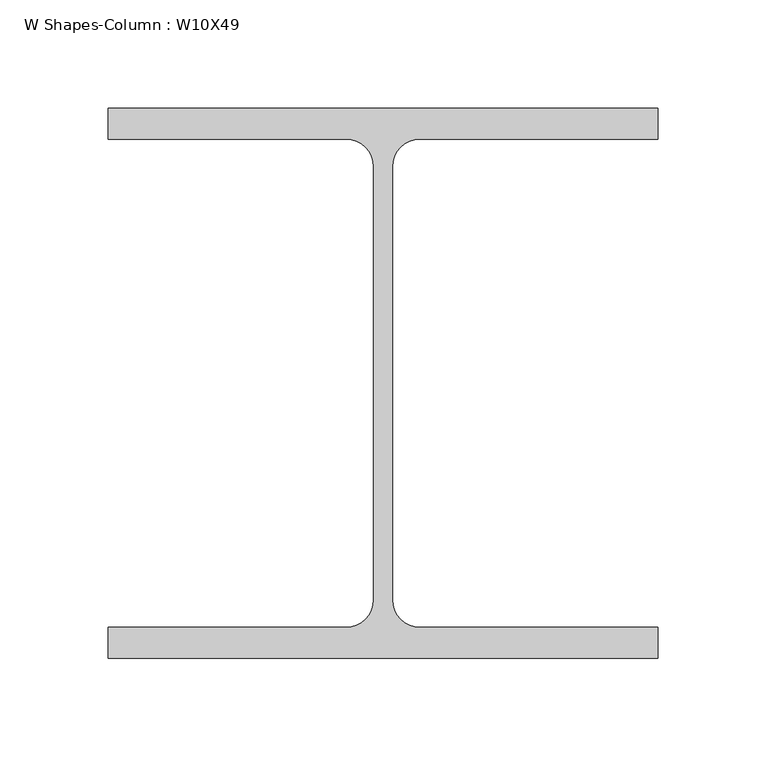
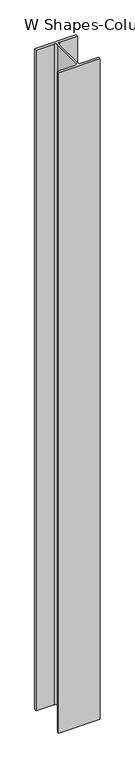
"""IFC4 building model written with IfcOpenShell, lengths in millimetres: column geometry, W Shapes-Column : W10X49."""

from ifc_helpers import new_model, si_unit, point, frame, frame_2d, origin, place, context, project, spatial, polyline, circle_curve, trimmed, segment, composite_curve, outline, extrude, source, transform, mapped, element, save


def w_shapes_column_w10x49_6b2d3d6a(model_context):
    return source(origin(), model_context, "Body", "SweptSolid", [
        extrude(outline(composite_curve([segment(polyline([(127.0, 127.0), (127.0, 112.776), (17.018, 112.776)]), True, "CONTINUOUS"), segment(trimmed(circle_curve(frame_2d((17.018, 100.076)), 12.7), [point((17.018, 112.776))], [point((4.318, 100.076))], True, "CARTESIAN"), True, "CONTINUOUS"), segment(polyline([(4.318, 100.076), (4.318, -100.076)]), True, "CONTINUOUS"), segment(trimmed(circle_curve(frame_2d((17.018, -100.076)), 12.7), [point((4.318, -100.076))], [point((17.018, -112.776))], True, "CARTESIAN"), True, "CONTINUOUS"), segment(polyline([(17.018, -112.776), (127.0, -112.776), (127.0, -127.0), (-127.0, -127.0), (-127.0, -112.776), (-17.018, -112.776)]), True, "CONTINUOUS"), segment(trimmed(circle_curve(frame_2d((-17.018, -100.076)), 12.7), [point((-17.018, -112.776))], [point((-4.318, -100.076))], True, "CARTESIAN"), True, "CONTINUOUS"), segment(polyline([(-4.318, -100.076), (-4.318, 100.076)]), True, "CONTINUOUS"), segment(trimmed(circle_curve(frame_2d((-17.018, 100.076)), 12.7), [point((-4.318, 100.076))], [point((-17.018, 112.776))], True, "CARTESIAN"), True, "CONTINUOUS"), segment(polyline([(-17.018, 112.776), (-127.0, 112.776), (-127.0, 127.0), (127.0, 127.0)]), True, "CONTINUOUS")], self_intersect=False)), frame((0.0, 0.0, 4267.4), z_axis=(0.0, 0.0, 1.0), x_axis=(1.0, 0.0, 0.0)), (0.0, 0.0, 1.0), 4267.0),
    ])


if __name__ == "__main__":
    model = new_model("IFC4")
    model_context = context("Model", 3, world=origin())
    ifc_project = project(units=[si_unit("LENGTHUNIT", "METRE", prefix="MILLI")], contexts=[model_context])
    site = spatial("IfcSite", under=ifc_project)
    building = spatial("IfcBuilding", under=site)
    placement = place(None, origin())
    w_shapes_column_w10x49_shape = w_shapes_column_w10x49_6b2d3d6a(model_context)
    element("IfcColumn", 1, ObjectType="W Shapes-Column : W10X49", at=placement, inside=building, context=model_context, shape_type="MappedRepresentation", body=[
        mapped(w_shapes_column_w10x49_shape, transform((0.0, 0.0, 0.0), x_axis=(1.0, 0.0, 0.0), y_axis=(0.0, 1.0, 0.0), z_axis=(0.0, 0.0, 1.0))),
    ])
    save(model, "model.ifc")

# Revit data of these elements
# Type "W Shapes-Column : W10X49"
#   Section Name Key = "W10X49"
#   Width = 10.000"
#   Web Thickness = 0.340"
#   Web Fillet = 0.500"
#   Warping Constant = 2070.00 in⁶
#   Torsional Moment of Inertia = 1.39 in⁴
#   Section Area = 14.40 in²
#   Plastic Modulus weak axis = 28.30 in³
#   Plastic Modulus strong axis = 60.40 in³
#   Perimeter = 4.875 ft²/ft
#   Nominal Weight = 49.00 lbf/ft
#   Moment of Inertia weak axis = 93.40 in⁴
#   Moment of Inertia strong axis = 272.00 in⁴
#   Height = 10.000"
#   Flange Thickness = 0.560"
#   Elastic Modulus weak axis = 18.70 in³
#   Elastic Modulus strong axis = 54.60 in³
#   Clear Web Height = 0' - 7 1/2"
#   Centroid Vertical = 5.000"
#   Centroid Horizontal = 5.000"
#   Bolt Spacing = 0' - 5 1/2"
#   Structural Material [instance default] = Steel ASTM A992
#   Principal Axes Angle = 0
# Element 1 (IfcColumn, "W Shapes-Column : W10X49")
#   Materials on its faces: "Steel ASTM A992"
# Materials
#   "Steel ASTM A992": class "Metal", colour RGB 199 199 199, transparency 0, Description = "Structural steel 50ksi", Cost = 0
